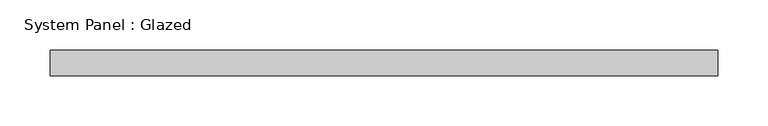
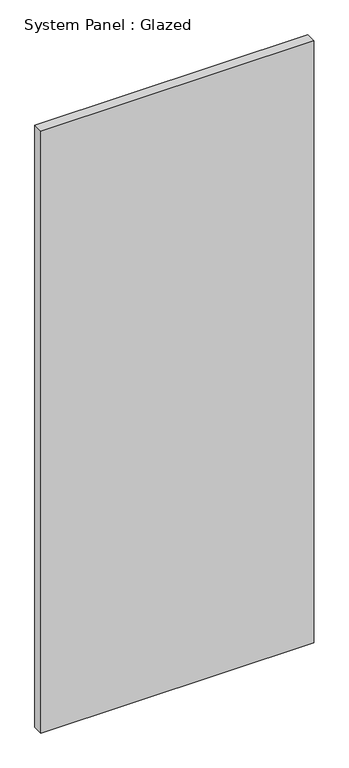
"""IFC4 building model written with IfcOpenShell, lengths in millimetres: plate geometry, System Panel : Glazed."""

from ifc_helpers import new_model, si_unit, origin, origin_with_axes, place, context, project, spatial, polyline, outline, extrude, source, transform, mapped, element, save


def system_panel_glazed_7de79e50(model_context):
    return source(origin(), model_context, "Body", "SweptSolid", [
        extrude(outline(polyline([(333.375, 19.05), (-333.375, 19.05), (-333.375, 44.45), (333.375, 44.45), (333.375, 19.05)])), origin_with_axes(), (0.0, 0.0, 1.0), 1553.4980219),
    ])


if __name__ == "__main__":
    model = new_model("IFC4")
    model_context = context("Model", 3, world=origin())
    ifc_project = project(units=[si_unit("LENGTHUNIT", "METRE", prefix="MILLI")], contexts=[model_context])
    site = spatial("IfcSite", under=ifc_project)
    building = spatial("IfcBuilding", under=site)
    placement = place(None, origin())
    system_panel_glazed_shape = system_panel_glazed_7de79e50(model_context)
    element("IfcPlate", 1, ObjectType="System Panel : Glazed", at=placement, inside=building, context=model_context, shape_type="MappedRepresentation", body=[
        mapped(system_panel_glazed_shape, transform((0.0, 0.0, 0.0), x_axis=(1.0, 0.0, 0.0), y_axis=(0.0, 1.0, 0.0), z_axis=(0.0, 0.0, 1.0))),
    ])
    save(model, "model.ifc")

# Revit data of these elements
# Type "System Panel : Glazed"
#   Construction Type Id = "GSP4R"
#   Analytic Construction = "1/8 in Pilkington single glazing"
#   Visual Light Transmittance = 0.9
#   Solar Heat Gain Coefficient = 0.86
#   Heat Transfer Coefficient (U) = 1.18115 BTU/(h·ft²·°F)
#   Define Thermal Properties by = 1
# Element 1 (IfcPlate, "System Panel : Glazed")
#   Materials on its faces: "Glass"
# Materials
#   "Glass": class "Glass", colour RGB 0 128 192, transparency 0.75, Description = "Soda Lime Glass", Cost = 0
